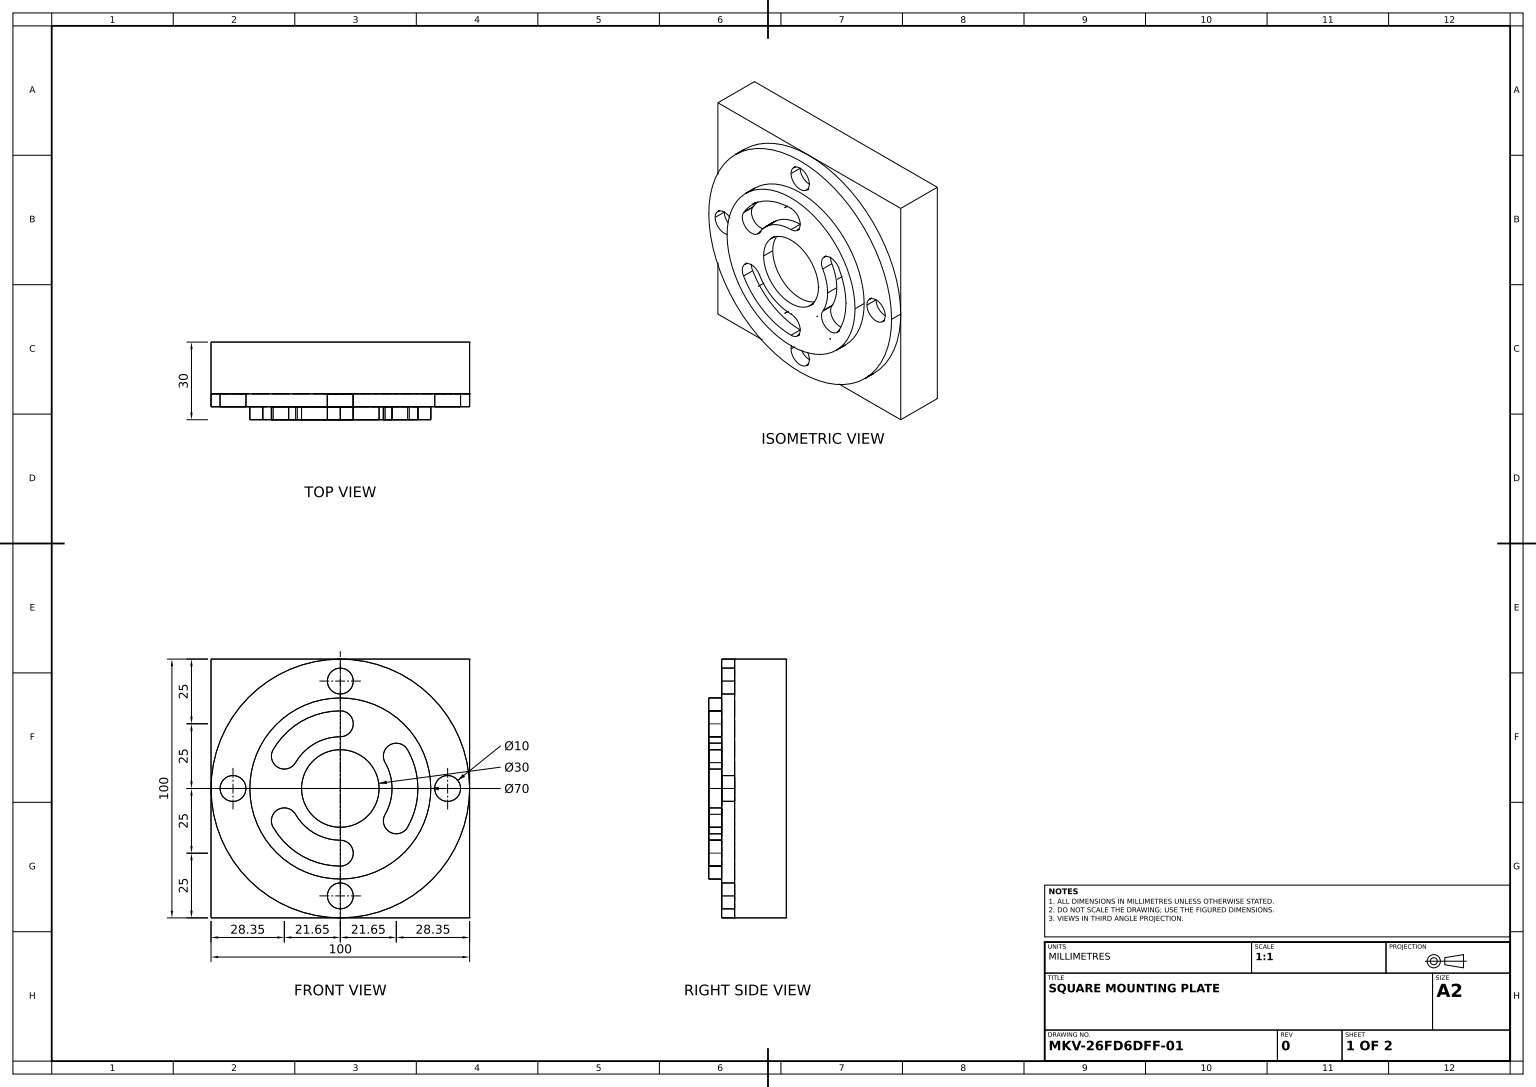
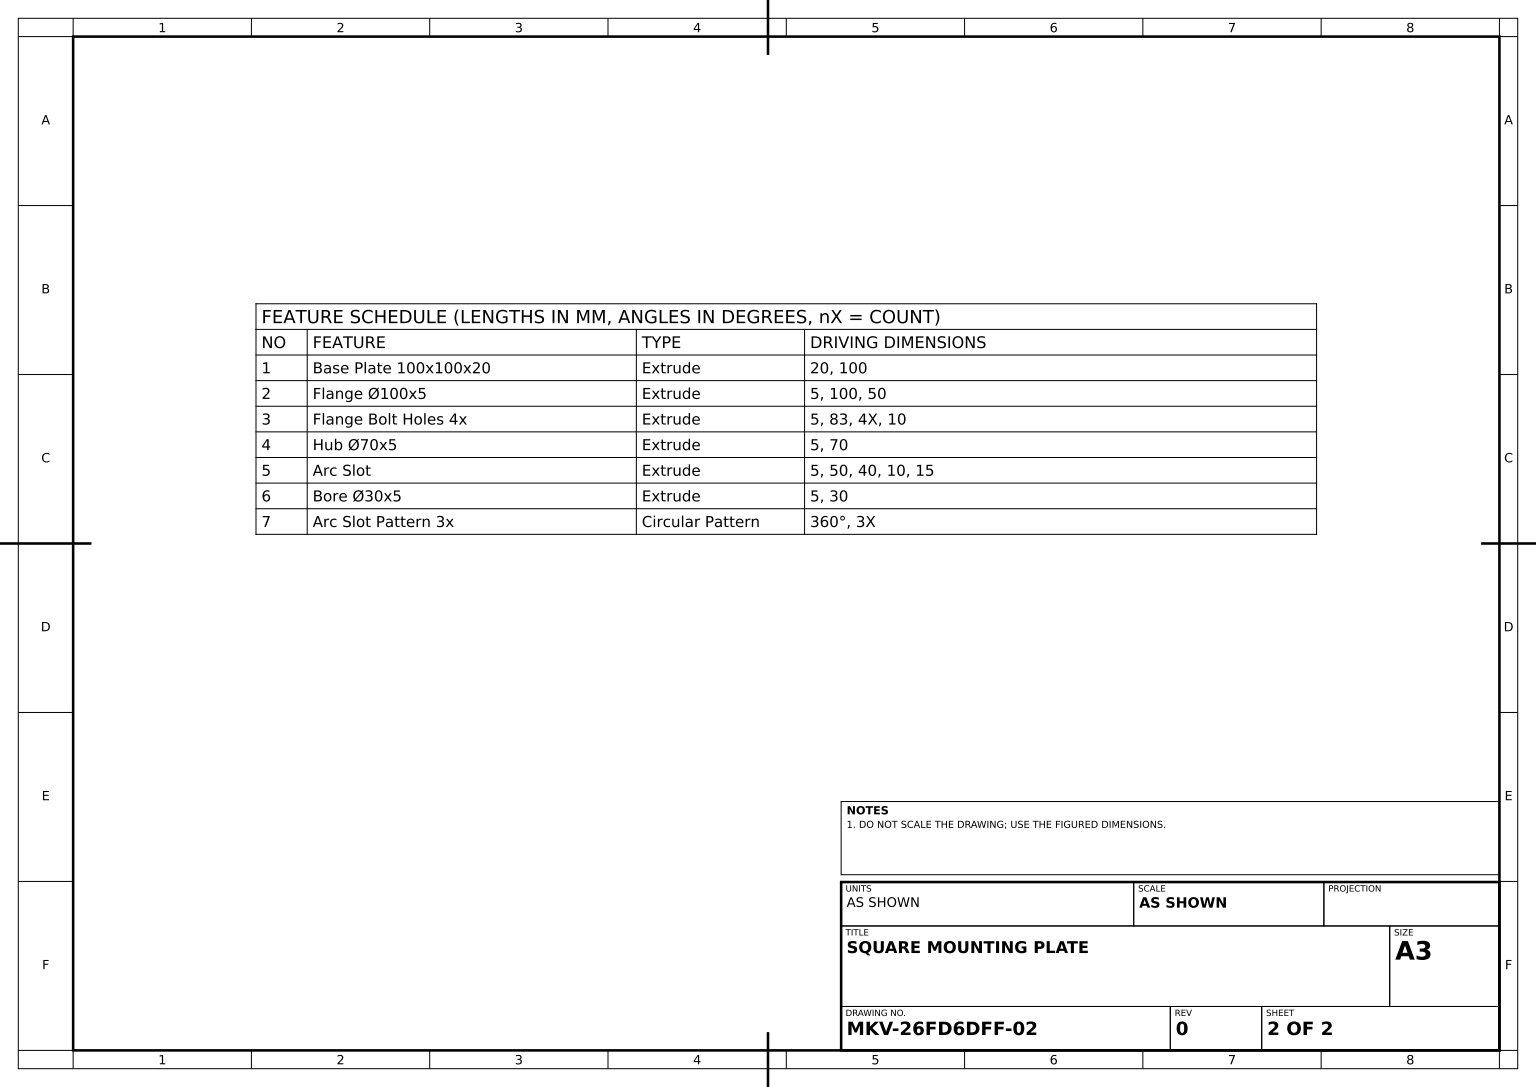
from build123d import *

# Parameters (mm, degrees)
BASE_PLATE_SKETCH_W         = 100
BASE_PLATE_SKETCH_H         = 100
BASE_PLATE_100X100X20_DEPTH = 20
FLANGE_SKETCH_R             = 50
FLANGE_100X5_DEPTH          = 5
FLANGE_BOLT_HOLES_SKETCH_R  = 5
FLANGE_BOLT_HOLES_4X_DEPTH  = 5
HUB_SKETCH_R                = 35
HUB_70X5_DEPTH              = 5
ARC_SLOT_DEPTH              = 5
BORE_SKETCH_R               = 15
BORE_30X5_DEPTH             = 5
ARC_SLOT_PATTERN_3X_COUNT   = 3


with BuildPart() as part:
    # Base Plate Sketch → Base Plate 100x100x20 (new body)
    with BuildSketch(Plane.XY):
        with Locations((50, 50)):
            Rectangle(BASE_PLATE_SKETCH_W, BASE_PLATE_SKETCH_H)
    extrude(amount=BASE_PLATE_100X100X20_DEPTH)

    # Flange Sketch → Flange Ø100x5 (add)
    with BuildSketch(Plane.XY.offset(20)):
        with Locations((50, 50)):
            Circle(FLANGE_SKETCH_R)
    extrude(amount=FLANGE_100X5_DEPTH)

    # Flange Bolt Holes Sketch → Flange Bolt Holes 4x (cut)
    with BuildSketch(Plane.XY.offset(25)):
        with Locations((50, 91.5)):
            Circle(FLANGE_BOLT_HOLES_SKETCH_R)
        with Locations((91.5, 50)):
            Circle(FLANGE_BOLT_HOLES_SKETCH_R)
        with Locations((50, 8.5)):
            Circle(FLANGE_BOLT_HOLES_SKETCH_R)
        with Locations((8.5, 50)):
            Circle(FLANGE_BOLT_HOLES_SKETCH_R)
    extrude(amount=-FLANGE_BOLT_HOLES_4X_DEPTH, mode=Mode.SUBTRACT)

    # Hub Sketch → Hub Ø70x5 (add)
    with BuildSketch(Plane.XY.offset(25)):
        with Locations((50, 50)):
            Circle(HUB_SKETCH_R)
    extrude(amount=HUB_70X5_DEPTH)

    # Arc Slot Sketch → Arc Slot (cut)
    with BuildSketch(Plane.XY.offset(30)):
        with BuildLine():
            ThreePointArc((50, 70), (40, 67.320508076), (32.679491924, 60))
            ThreePointArc((32.679491924, 60), (25.849364905, 58.169872981), (24.019237886, 65))
            ThreePointArc((24.019237886, 65), (35, 75.980762114), (50, 80))
            ThreePointArc((50, 80), (55, 75), (50, 70))
        make_face()
    arc_slot = extrude(amount=-ARC_SLOT_DEPTH, mode=Mode.SUBTRACT)

    # Bore Sketch → Bore Ø30x5 (cut)
    with BuildSketch(Plane.XY.offset(30)):
        with Locations((50, 50)):
            Circle(BORE_SKETCH_R)
    extrude(amount=-BORE_30X5_DEPTH, mode=Mode.SUBTRACT)

    # Arc Slot Pattern 3x: Arc Slot ×3 about axis
    arc_slot_pattern_3x_axis = Axis((50, 50, 0), (0, 0, 1))
    for i in range(1, ARC_SLOT_PATTERN_3X_COUNT):
        add(arc_slot.rotate(arc_slot_pattern_3x_axis, i * 360 / ARC_SLOT_PATTERN_3X_COUNT), mode=Mode.SUBTRACT)


solid = part.part
